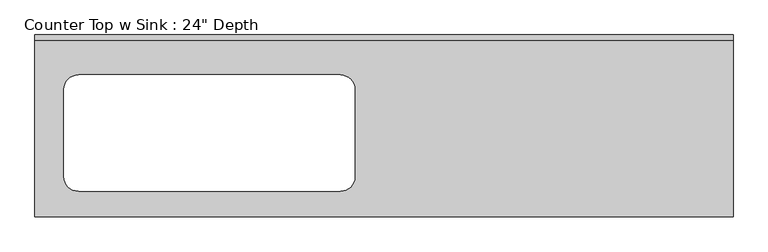
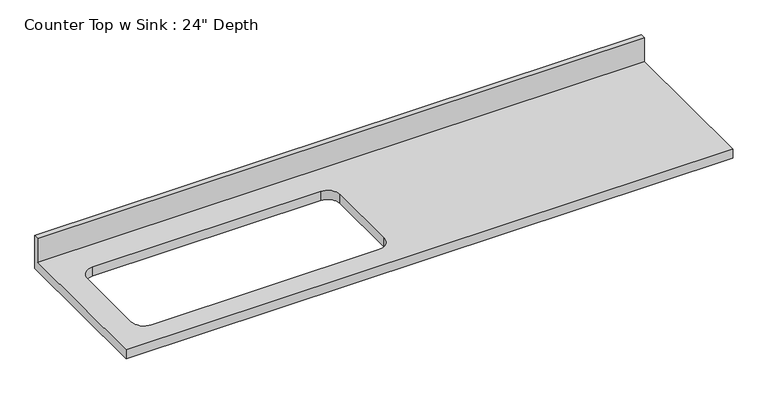
"""IFC4 building model written with IfcOpenShell, lengths in millimetres: furniture geometry."""

from ifc_helpers import new_model, si_unit, frame, origin, place, context, project, spatial, polyline, circle_curve, source, transform, mapped, element, save
from ifc_brep_helpers import plane_surface, revolved_surface, advanced_brep


def furniture_91b07d4a(model_context):
    return source(origin(), model_context, "Body", "AdvancedBrep", [
        advanced_brep(
        [(-1200.4622951, -635.0, 914.4), (1237.9377049, -635.0, 914.4), (1237.9377049, -19.05, 914.4), (-1200.4622951, -19.05, 914.4), (-1048.0622951, -139.7, 914.4), (-133.6622951, -139.7, 914.4), (-82.8622951, -190.5, 914.4), (-82.8622951, -495.3, 914.4), (-133.6622951, -546.1, 914.4), (-1048.0622951, -546.1, 914.4), (-1098.8622951, -495.3, 914.4), (-1098.8622951, -190.5, 914.4), (1237.9377049, 0.0, 876.3), (1237.9377049, -635.0, 876.3), (-1200.4622951, -635.0, 876.3), (-1200.4622951, 0.0, 876.3), (-133.6622951, -139.7, 876.3), (-1048.0622951, -139.7, 876.3), (-1098.8622951, -190.5, 876.3), (-1098.8622951, -495.3, 876.3), (-1048.0622951, -546.1, 876.3), (-133.6622951, -546.1, 876.3), (-82.8622951, -495.3, 876.3), (-82.8622951, -190.5, 876.3), (-1200.4622951, 0.0, 1016.0), (1237.9377049, 0.0, 1016.0), (-1200.4622951, -19.05, 1016.0), (1237.9377049, -19.05, 1016.0)],
        [
            (0, 1),
            (1, 2),
            (2, 3),
            (3, 0),
            (4, 5),
            (5, 6, circle_curve(frame((-133.6622951, -190.5, 914.4), z_axis=(0.0, 0.0, -1.0), x_axis=(1.0, 0.0, 0.0)), 50.8)),
            (6, 7),
            (7, 8, circle_curve(frame((-133.6622951, -495.3, 914.4), z_axis=(0.0, 0.0, -1.0), x_axis=(1.0, 0.0, 0.0)), 50.8)),
            (8, 9),
            (9, 10, circle_curve(frame((-1048.0622951, -495.3, 914.4), z_axis=(0.0, 0.0, -1.0), x_axis=(1.0, 0.0, 0.0)), 50.8)),
            (10, 11),
            (11, 4, circle_curve(frame((-1048.0622951, -190.5, 914.4), z_axis=(0.0, 0.0, -1.0), x_axis=(1.0, 0.0, 0.0)), 50.8)),
            (12, 13),
            (13, 14),
            (14, 15),
            (15, 12),
            (16, 17),
            (17, 18, circle_curve(frame((-1048.0622951, -190.5, 876.3), z_axis=(0.0, 0.0, 1.0), x_axis=(1.0, 0.0, 0.0)), 50.8)),
            (18, 19),
            (19, 20, circle_curve(frame((-1048.0622951, -495.3, 876.3), z_axis=(0.0, 0.0, 1.0), x_axis=(1.0, 0.0, 0.0)), 50.8)),
            (20, 21),
            (21, 22, circle_curve(frame((-133.6622951, -495.3, 876.3), z_axis=(0.0, 0.0, 1.0), x_axis=(1.0, 0.0, 0.0)), 50.8)),
            (22, 23),
            (23, 16, circle_curve(frame((-133.6622951, -190.5, 876.3), z_axis=(0.0, 0.0, 1.0), x_axis=(1.0, 0.0, 0.0)), 50.8)),
            (15, 24),
            (24, 25),
            (25, 12),
            (14, 0),
            (3, 26),
            (26, 24),
            (13, 1),
            (25, 27),
            (27, 2),
            (26, 27),
            (4, 17),
            (16, 5),
            (11, 18),
            (10, 19),
            (9, 20),
            (8, 21),
            (7, 22),
            (6, 23),
        ],
        [
            plane_surface(frame((-1200.4622951, 0.0, 914.4), z_axis=(0.0, 0.0, 1.0), x_axis=(-1.0, 0.0, 0.0))),
            plane_surface(frame((-1200.4622951, 0.0, 876.3), z_axis=(0.0, 0.0, -1.0), x_axis=(1.0, 0.0, 0.0))),
            plane_surface(frame((1237.9377049, 0.0, 914.4), z_axis=(0.0, 1.0, 0.0), x_axis=(0.0, 0.0, -1.0))),
            plane_surface(frame((-1200.4622951, 0.0, 914.4), z_axis=(-1.0, 0.0, 0.0), x_axis=(0.0, 0.0, -1.0))),
            plane_surface(frame((-1200.4622951, -635.0, 914.4), z_axis=(0.0, -1.0, 0.0), x_axis=(0.0, 0.0, -1.0))),
            plane_surface(frame((1237.9377049, -635.0, 914.4), z_axis=(1.0, 0.0, 0.0), x_axis=(0.0, 0.0, -1.0))),
            plane_surface(frame((-1200.4622951, 0.0, 1016.0), z_axis=(0.0, 0.0, 1.0), x_axis=(0.0, -1.0, 0.0))),
            plane_surface(frame((-1200.4622951, -19.05, 1016.0), z_axis=(0.0, -1.0, 0.0), x_axis=(0.0, 0.0, -1.0))),
            plane_surface(frame((-133.6622951, -139.7, 914.4), z_axis=(0.0, -1.0, 0.0), x_axis=(0.0, 0.0, -1.0))),
            revolved_surface(polyline([(-997.2622951000001, -190.5, 914.4), (-997.2622951000001, -190.5, 876.3)]), (-1048.0622951, -190.5, 876.3), (0.0, 0.0, 1.0)),
            plane_surface(frame((-1098.8622951, -190.5, 914.4), z_axis=(1.0, 0.0, 0.0), x_axis=(0.0, 0.0, -1.0))),
            revolved_surface(polyline([(-997.2622951000001, -495.3, 914.4), (-997.2622951000001, -495.3, 876.3)]), (-1048.0622951, -495.3, 876.3), (0.0, 0.0, 1.0)),
            plane_surface(frame((-1048.0622951, -546.1, 914.4), z_axis=(0.0, 1.0, 0.0), x_axis=(0.0, 0.0, -1.0))),
            revolved_surface(polyline([(-82.8622951, -495.3, 914.4), (-82.8622951, -495.3, 876.3)]), (-133.6622951, -495.3, 876.3), (0.0, 0.0, 1.0)),
            plane_surface(frame((-82.8622951, -495.3, 914.4), z_axis=(-1.0, 0.0, 0.0), x_axis=(0.0, 0.0, -1.0))),
            revolved_surface(polyline([(-82.8622951, -190.5, 914.4), (-82.8622951, -190.5, 876.3)]), (-133.6622951, -190.5, 876.3), (0.0, 0.0, 1.0)),
        ],
        [
            (0, [[1, 2, 3, 4], [5, 6, 7, 8, 9, 10, 11, 12]]),
            (1, [[13, 14, 15, 16], [17, 18, 19, 20, 21, 22, 23, 24]]),
            (2, [[-16, 25, 26, 27]]),
            (3, [[-15, 28, -4, 29, 30, -25]]),
            (4, [[-1, -28, -14, 31]]),
            (5, [[-13, -27, 32, 33, -2, -31]]),
            (6, [[-30, 34, -32, -26]]),
            (7, [[-34, -29, -3, -33]]),
            (8, [[35, -17, 36, -5]]),
            (9, [[-35, -12, 37, -18]]),
            (10, [[-37, -11, 38, -19]]),
            (11, [[-38, -10, 39, -20]]),
            (12, [[-39, -9, 40, -21]]),
            (13, [[-40, -8, 41, -22]]),
            (14, [[-41, -7, 42, -23]]),
            (15, [[-36, -24, -42, -6]]),
        ],
    ),
    ])


if __name__ == "__main__":
    model = new_model("IFC4")
    model_context = context("Model", 3, world=origin())
    ifc_project = project(units=[si_unit("LENGTHUNIT", "METRE", prefix="MILLI")], contexts=[model_context])
    site = spatial("IfcSite", under=ifc_project)
    building = spatial("IfcBuilding", under=site)
    placement = place(None, origin())
    furniture_shape = furniture_91b07d4a(model_context)
    element("IfcFurniture", 1, ObjectType="Counter Top w Sink : 24\" Depth", at=placement, inside=building, context=model_context, shape_type="MappedRepresentation", body=[
        mapped(furniture_shape, transform((0.0, 0.0, 0.0), x_axis=(1.0, 0.0, 0.0), y_axis=(0.0, 1.0, 0.0), z_axis=(0.0, 0.0, 1.0))),
    ])
    save(model, "model.ifc")

# Revit data of these elements
# Type "Counter Top w Sink : 24\" Depth"
#   Assembly Code = "C1030400"
#   Counter Thickness = 0' - 1 1/2"
#   Depth = 2' - 1"
#   Height = 3' - 0"
#   Length [instance default] = 8' - 0"
#   Sink Location [instance default] = 2' - 0"
#   Sink Location To Wall [instance default] = 0' - 6"
#   Sink Opening Depth [instance default] = 1' - 3"
#   Sink Opening Width [instance default] = 3' - 3"
#   Counter Top Material = none
#   Default Elevation = 0
# Element 1 (IfcFurniture, "Counter Top w Sink : 24\" Depth")
#   Materials on its faces: "Counter Top"
# Materials
#   "Counter Top": class "Wood", colour RGB 226 177 128, transparency 0
